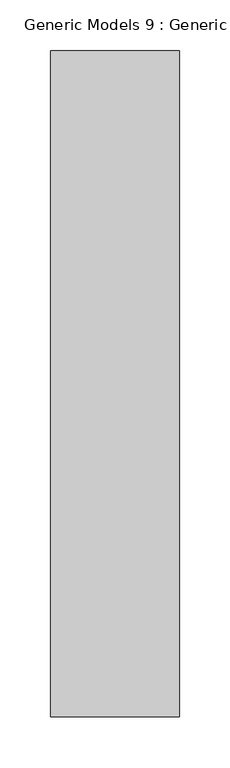
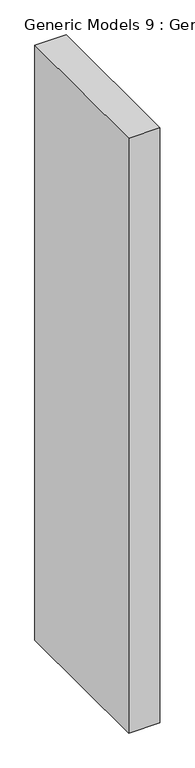
"""IFC4 building model written with IfcOpenShell, lengths in millimetres: proxy geometry, Generic Models 9 : Generic Models 9."""

from ifc_helpers import new_model, si_unit, frame, origin, place, context, project, spatial, polyline, outline, extrude, source, transform, mapped, element, save


def generic_models_9_generic_models_9_50e4b17c(model_context):
    return source(origin(), model_context, "Body", "SweptSolid", [
        extrude(outline(polyline([(1022.326752, -3772.4866303), (895.326752, -3772.4866303), (895.326752, -3115.8874941), (1022.326752, -3115.8874941), (1022.326752, -3772.4866303)])), frame((0.0, 0.0, 3563.2571429), z_axis=(0.0, 0.0, 1.0), x_axis=(1.0, 0.0, 0.0)), (0.0, 0.0, 1.0), 2545.662837),
    ])


if __name__ == "__main__":
    model = new_model("IFC4")
    model_context = context("Model", 3, world=origin())
    ifc_project = project(units=[si_unit("LENGTHUNIT", "METRE", prefix="MILLI")], contexts=[model_context])
    site = spatial("IfcSite", under=ifc_project)
    building = spatial("IfcBuilding", under=site)
    placement = place(None, origin())
    generic_models_9_generic_models_9_shape = generic_models_9_generic_models_9_50e4b17c(model_context)
    element("IfcBuildingElementProxy", 1, Name="Generic Models 9 : Generic Models 9", ObjectType="Generic Models 9 : Generic Models 9", at=placement, inside=building, context=model_context, shape_type="MappedRepresentation", body=[
        mapped(generic_models_9_generic_models_9_shape, transform((0.0, 0.0, 0.0), x_axis=(1.0, 0.0, 0.0), y_axis=(0.0, 1.0, 0.0), z_axis=(0.0, 0.0, 1.0))),
    ])
    save(model, "model.ifc")

# Revit data of these elements
# Element 1 (IfcBuildingElementProxy, "Generic Models 9 : Generic Models 9")
#   Materials on its faces: "Clad - White"
# Materials
#   "Clad - White": class "Wood", colour RGB 242 242 238, transparency 0, Cost = 0
